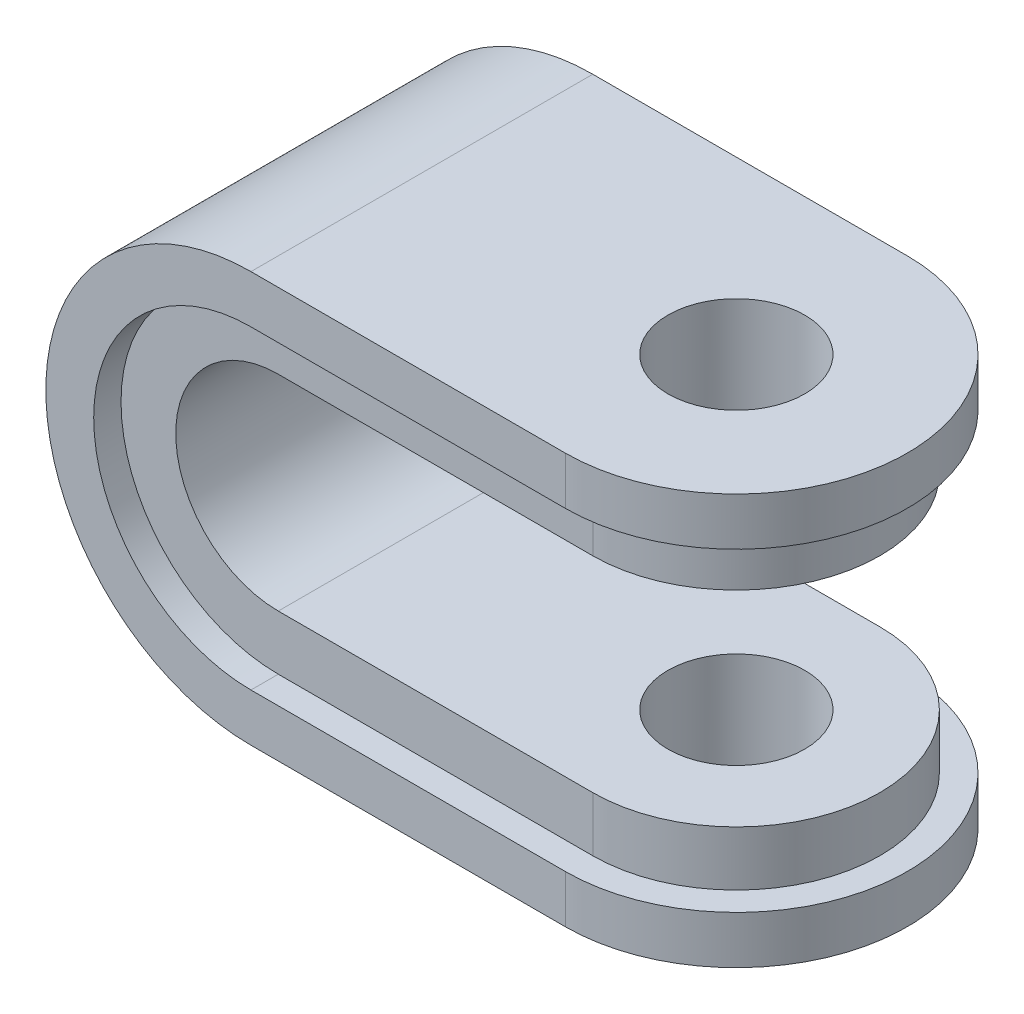
ISO-10303-21;
HEADER;
FILE_DESCRIPTION(('STEP AP214'),'2;1');
FILE_NAME('part.step','',(''),(''),'','','');
FILE_SCHEMA(('AUTOMOTIVE_DESIGN { 1 0 10303 214 1 1 1 1 }'));
ENDSEC;
DATA;
#1=APPLICATION_CONTEXT('core data for automotive mechanical design processes');
#2=APPLICATION_PROTOCOL_DEFINITION('international standard','automotive_design',2000,#1);
#3=PRODUCT_CONTEXT('',#1,'mechanical');
#4=PRODUCT('Part','Part','',(#3));
#5=PRODUCT_RELATED_PRODUCT_CATEGORY('part','',(#4));
#6=PRODUCT_DEFINITION_FORMATION('','',#4);
#7=PRODUCT_DEFINITION_CONTEXT('part definition',#1,'design');
#8=PRODUCT_DEFINITION('design','',#6,#7);
#9=PRODUCT_DEFINITION_SHAPE('','',#8);
#10=(LENGTH_UNIT() NAMED_UNIT(*) SI_UNIT(.MILLI.,.METRE.));
#11=(NAMED_UNIT(*) PLANE_ANGLE_UNIT() SI_UNIT($,.RADIAN.));
#12=(NAMED_UNIT(*) SI_UNIT($,.STERADIAN.) SOLID_ANGLE_UNIT());
#13=UNCERTAINTY_MEASURE_WITH_UNIT(LENGTH_MEASURE(1.E-05),#10,'distance_accuracy_value','');
#14=(GEOMETRIC_REPRESENTATION_CONTEXT(3) GLOBAL_UNCERTAINTY_ASSIGNED_CONTEXT((#13)) GLOBAL_UNIT_ASSIGNED_CONTEXT((#10,
#11,#12)) REPRESENTATION_CONTEXT('',''));
#15=CARTESIAN_POINT('',(0.,0.,0.));
#16=DIRECTION('',(0.,0.,1.));
#17=DIRECTION('',(1.,0.,0.));
#18=AXIS2_PLACEMENT_3D('',#15,#16,#17);
#19=CARTESIAN_POINT('',(46.,8.,25.));
#20=DIRECTION('',(0.,-1.,0.));
#21=DIRECTION('',(0.,0.,-1.));
#22=AXIS2_PLACEMENT_3D('',#19,#20,#21);
#23=CYLINDRICAL_SURFACE('',#22,25.);
#24=DIRECTION('',(0.,-1.,0.));
#25=VECTOR('',#24,1.);
#26=CARTESIAN_POINT('',(46.,0.,0.));
#27=LINE('',#26,#25);
#28=CARTESIAN_POINT('',(46.,7.,0.));
#29=VERTEX_POINT('',#28);
#30=CARTESIAN_POINT('',(46.,0.,0.));
#31=VERTEX_POINT('',#30);
#32=EDGE_CURVE('E179',#29,#31,#27,.T.);
#33=ORIENTED_EDGE('',*,*,#32,.F.);
#34=CARTESIAN_POINT('',(46.,7.,25.));
#35=DIRECTION('',(0.,1.,0.));
#36=DIRECTION('',(0.,0.,1.));
#37=AXIS2_PLACEMENT_3D('',#34,#35,#36);
#38=CIRCLE('',#37,25.);
#39=CARTESIAN_POINT('',(46.,6.99999999999999,50.));
#40=VERTEX_POINT('',#39);
#41=EDGE_CURVE('E222',#40,#29,#38,.T.);
#42=ORIENTED_EDGE('',*,*,#41,.F.);
#43=DIRECTION('',(0.,-1.,0.));
#44=VECTOR('',#43,1.);
#45=CARTESIAN_POINT('',(46.,0.,50.));
#46=LINE('',#45,#44);
#47=CARTESIAN_POINT('',(46.,0.,50.));
#48=VERTEX_POINT('',#47);
#49=EDGE_CURVE('E187',#40,#48,#46,.T.);
#50=ORIENTED_EDGE('',*,*,#49,.T.);
#51=CARTESIAN_POINT('',(46.,0.,25.));
#52=DIRECTION('',(0.,-1.,0.));
#53=DIRECTION('',(0.,0.,-1.));
#54=AXIS2_PLACEMENT_3D('',#51,#52,#53);
#55=CIRCLE('',#54,25.);
#56=EDGE_CURVE('E225',#31,#48,#55,.T.);
#57=ORIENTED_EDGE('',*,*,#56,.F.);
#58=EDGE_LOOP('',(#33,#42,#50,#57));
#59=FACE_BOUND('',#58,.T.);
#60=ADVANCED_FACE('F56',(#59),#23,.T.);
#61=CARTESIAN_POINT('',(46.,52.,25.));
#62=DIRECTION('',(0.,1.,0.));
#63=DIRECTION('',(0.,0.,1.));
#64=AXIS2_PLACEMENT_3D('',#61,#62,#63);
#65=CYLINDRICAL_SURFACE('',#64,25.);
#66=DIRECTION('',(0.,-1.,0.));
#67=VECTOR('',#66,1.);
#68=CARTESIAN_POINT('',(46.,0.,50.));
#69=LINE('',#68,#67);
#70=CARTESIAN_POINT('',(46.,60.,50.));
#71=VERTEX_POINT('',#70);
#72=CARTESIAN_POINT('',(46.,53.,50.));
#73=VERTEX_POINT('',#72);
#74=EDGE_CURVE('E176',#71,#73,#69,.T.);
#75=ORIENTED_EDGE('',*,*,#74,.T.);
#76=CARTESIAN_POINT('',(46.,53.,25.));
#77=DIRECTION('',(0.,-1.,0.));
#78=DIRECTION('',(0.,0.,-1.));
#79=AXIS2_PLACEMENT_3D('',#76,#77,#78);
#80=CIRCLE('',#79,25.);
#81=CARTESIAN_POINT('',(46.,53.,0.));
#82=VERTEX_POINT('',#81);
#83=EDGE_CURVE('E639',#82,#73,#80,.T.);
#84=ORIENTED_EDGE('',*,*,#83,.F.);
#85=DIRECTION('',(0.,-1.,0.));
#86=VECTOR('',#85,1.);
#87=CARTESIAN_POINT('',(46.,0.,0.));
#88=LINE('',#87,#86);
#89=CARTESIAN_POINT('',(46.,60.,0.));
#90=VERTEX_POINT('',#89);
#91=EDGE_CURVE('E172',#90,#82,#88,.T.);
#92=ORIENTED_EDGE('',*,*,#91,.F.);
#93=CARTESIAN_POINT('',(46.,60.,25.));
#94=DIRECTION('',(0.,1.,0.));
#95=DIRECTION('',(0.,0.,1.));
#96=AXIS2_PLACEMENT_3D('',#93,#94,#95);
#97=CIRCLE('',#96,25.);
#98=EDGE_CURVE('E306',#71,#90,#97,.T.);
#99=ORIENTED_EDGE('',*,*,#98,.F.);
#100=EDGE_LOOP('',(#75,#84,#92,#99));
#101=FACE_BOUND('',#100,.T.);
#102=ADVANCED_FACE('F349',(#101),#65,.T.);
#103=CARTESIAN_POINT('',(46.,7.,25.));
#104=DIRECTION('',(0.,1.,0.));
#105=DIRECTION('',(0.,0.,1.));
#106=AXIS2_PLACEMENT_3D('',#103,#104,#105);
#107=CYLINDRICAL_SURFACE('',#106,21.);
#108=CARTESIAN_POINT('',(46.,15.,25.));
#109=DIRECTION('',(0.,1.,0.));
#110=DIRECTION('',(0.,0.,1.));
#111=AXIS2_PLACEMENT_3D('',#108,#109,#110);
#112=CIRCLE('',#111,21.);
#113=CARTESIAN_POINT('',(46.,15.,46.));
#114=VERTEX_POINT('',#113);
#115=CARTESIAN_POINT('',(46.,15.,4.));
#116=VERTEX_POINT('',#115);
#117=EDGE_CURVE('E303',#114,#116,#112,.T.);
#118=ORIENTED_EDGE('',*,*,#117,.F.);
#119=DIRECTION('',(0.,1.,0.));
#120=VECTOR('',#119,1.);
#121=CARTESIAN_POINT('',(46.,6.99999999999999,46.));
#122=LINE('',#121,#120);
#123=CARTESIAN_POINT('',(46.,7.,46.));
#124=VERTEX_POINT('',#123);
#125=EDGE_CURVE('E163',#124,#114,#122,.T.);
#126=ORIENTED_EDGE('',*,*,#125,.F.);
#127=CARTESIAN_POINT('',(46.,7.,25.));
#128=DIRECTION('',(0.,-1.,0.));
#129=DIRECTION('',(0.,0.,1.));
#130=AXIS2_PLACEMENT_3D('',#127,#128,#129);
#131=CIRCLE('',#130,21.);
#132=CARTESIAN_POINT('',(46.,7.,4.));
#133=VERTEX_POINT('',#132);
#134=EDGE_CURVE('E328',#133,#124,#131,.T.);
#135=ORIENTED_EDGE('',*,*,#134,.F.);
#136=DIRECTION('',(0.,-1.,0.));
#137=VECTOR('',#136,1.);
#138=CARTESIAN_POINT('',(46.,6.99999999999999,4.));
#139=LINE('',#138,#137);
#140=EDGE_CURVE('E317',#116,#133,#139,.T.);
#141=ORIENTED_EDGE('',*,*,#140,.F.);
#142=EDGE_LOOP('',(#118,#126,#135,#141));
#143=FACE_BOUND('',#142,.T.);
#144=ADVANCED_FACE('F332',(#143),#107,.T.);
#145=CARTESIAN_POINT('',(46.,53.,25.));
#146=DIRECTION('',(0.,-1.,0.));
#147=DIRECTION('',(0.,0.,-1.));
#148=AXIS2_PLACEMENT_3D('',#145,#146,#147);
#149=CYLINDRICAL_SURFACE('',#148,21.);
#150=CARTESIAN_POINT('',(46.,45.,25.));
#151=DIRECTION('',(0.,-1.,0.));
#152=DIRECTION('',(0.,0.,-1.));
#153=AXIS2_PLACEMENT_3D('',#150,#151,#152);
#154=CIRCLE('',#153,21.);
#155=CARTESIAN_POINT('',(46.,45.,4.));
#156=VERTEX_POINT('',#155);
#157=CARTESIAN_POINT('',(46.,45.,46.));
#158=VERTEX_POINT('',#157);
#159=EDGE_CURVE('E299',#156,#158,#154,.T.);
#160=ORIENTED_EDGE('',*,*,#159,.F.);
#161=DIRECTION('',(0.,-1.,0.));
#162=VECTOR('',#161,1.);
#163=CARTESIAN_POINT('',(46.,53.,4.));
#164=LINE('',#163,#162);
#165=CARTESIAN_POINT('',(46.,53.,4.));
#166=VERTEX_POINT('',#165);
#167=EDGE_CURVE('E288',#166,#156,#164,.T.);
#168=ORIENTED_EDGE('',*,*,#167,.F.);
#169=CARTESIAN_POINT('',(46.,53.,25.));
#170=DIRECTION('',(0.,1.,0.));
#171=DIRECTION('',(0.,0.,-1.));
#172=AXIS2_PLACEMENT_3D('',#169,#170,#171);
#173=CIRCLE('',#172,21.);
#174=CARTESIAN_POINT('',(46.,53.,46.));
#175=VERTEX_POINT('',#174);
#176=EDGE_CURVE('E297',#175,#166,#173,.T.);
#177=ORIENTED_EDGE('',*,*,#176,.F.);
#178=DIRECTION('',(0.,1.,0.));
#179=VECTOR('',#178,1.);
#180=CARTESIAN_POINT('',(46.,53.,46.));
#181=LINE('',#180,#179);
#182=EDGE_CURVE('E152',#158,#175,#181,.T.);
#183=ORIENTED_EDGE('',*,*,#182,.F.);
#184=EDGE_LOOP('',(#160,#168,#177,#183));
#185=FACE_BOUND('',#184,.T.);
#186=ADVANCED_FACE('F296',(#185),#149,.T.);
#187=CARTESIAN_POINT('',(0.,45.,0.));
#188=DIRECTION('',(0.,-1.,0.));
#189=DIRECTION('',(0.,0.,-1.));
#190=AXIS2_PLACEMENT_3D('',#187,#188,#189);
#191=PLANE('',#190);
#192=CARTESIAN_POINT('',(46.,45.,25.));
#193=DIRECTION('',(0.,-1.,0.));
#194=DIRECTION('',(0.,0.,-1.));
#195=AXIS2_PLACEMENT_3D('',#192,#193,#194);
#196=CIRCLE('',#195,10.);
#197=CARTESIAN_POINT('',(46.,45.,15.));
#198=VERTEX_POINT('',#197);
#199=EDGE_CURVE('E382',#198,#198,#196,.T.);
#200=ORIENTED_EDGE('',*,*,#199,.F.);
#201=EDGE_LOOP('',(#200));
#202=FACE_BOUND('',#201,.T.);
#203=ORIENTED_EDGE('',*,*,#159,.T.);
#204=DIRECTION('',(1.,0.,0.));
#205=VECTOR('',#204,1.);
#206=CARTESIAN_POINT('',(0.,45.,46.));
#207=LINE('',#206,#205);
#208=CARTESIAN_POINT('',(0.,45.,46.));
#209=VERTEX_POINT('',#208);
#210=EDGE_CURVE('E158',#209,#158,#207,.T.);
#211=ORIENTED_EDGE('',*,*,#210,.F.);
#212=DIRECTION('',(0.,0.,1.));
#213=VECTOR('',#212,1.);
#214=CARTESIAN_POINT('',(0.,45.,0.));
#215=LINE('',#214,#213);
#216=CARTESIAN_POINT('',(0.,45.,4.));
#217=VERTEX_POINT('',#216);
#218=EDGE_CURVE('E117',#217,#209,#215,.T.);
#219=ORIENTED_EDGE('',*,*,#218,.F.);
#220=DIRECTION('',(-1.,0.,0.));
#221=VECTOR('',#220,1.);
#222=CARTESIAN_POINT('',(46.,45.,4.));
#223=LINE('',#222,#221);
#224=EDGE_CURVE('E287',#156,#217,#223,.T.);
#225=ORIENTED_EDGE('',*,*,#224,.F.);
#226=EDGE_LOOP('',(#203,#211,#219,#225));
#227=FACE_BOUND('',#226,.T.);
#228=ADVANCED_FACE('F305',(#202,#227),#191,.T.);
#229=CARTESIAN_POINT('',(0.,30.,0.));
#230=DIRECTION('',(0.,0.,1.));
#231=DIRECTION('',(1.,0.,0.));
#232=AXIS2_PLACEMENT_3D('',#229,#230,#231);
#233=CYLINDRICAL_SURFACE('',#232,15.);
#234=DIRECTION('',(0.,0.,1.));
#235=VECTOR('',#234,1.);
#236=CARTESIAN_POINT('',(0.,15.,0.));
#237=LINE('',#236,#235);
#238=CARTESIAN_POINT('',(0.,15.,4.));
#239=VERTEX_POINT('',#238);
#240=CARTESIAN_POINT('',(0.,15.,46.));
#241=VERTEX_POINT('',#240);
#242=EDGE_CURVE('E92',#239,#241,#237,.T.);
#243=ORIENTED_EDGE('',*,*,#242,.F.);
#244=CARTESIAN_POINT('',(0.,30.,4.));
#245=DIRECTION('',(0.,0.,1.));
#246=DIRECTION('',(-1.,0.,0.));
#247=AXIS2_PLACEMENT_3D('',#244,#245,#246);
#248=CIRCLE('',#247,15.);
#249=EDGE_CURVE('E311',#217,#239,#248,.T.);
#250=ORIENTED_EDGE('',*,*,#249,.F.);
#251=ORIENTED_EDGE('',*,*,#218,.T.);
#252=CARTESIAN_POINT('',(0.,30.,46.));
#253=DIRECTION('',(0.,0.,-1.));
#254=DIRECTION('',(1.,0.,0.));
#255=AXIS2_PLACEMENT_3D('',#252,#253,#254);
#256=CIRCLE('',#255,15.);
#257=EDGE_CURVE('E171',#241,#209,#256,.T.);
#258=ORIENTED_EDGE('',*,*,#257,.F.);
#259=EDGE_LOOP('',(#243,#250,#251,#258));
#260=FACE_BOUND('',#259,.T.);
#261=ADVANCED_FACE('F337',(#260),#233,.F.);
#262=CARTESIAN_POINT('',(0.,15.,0.));
#263=DIRECTION('',(0.,1.,0.));
#264=DIRECTION('',(0.,0.,1.));
#265=AXIS2_PLACEMENT_3D('',#262,#263,#264);
#266=PLANE('',#265);
#267=CARTESIAN_POINT('',(46.,15.,25.));
#268=DIRECTION('',(0.,1.,0.));
#269=DIRECTION('',(0.,0.,1.));
#270=AXIS2_PLACEMENT_3D('',#267,#268,#269);
#271=CIRCLE('',#270,10.);
#272=CARTESIAN_POINT('',(46.,15.,35.));
#273=VERTEX_POINT('',#272);
#274=EDGE_CURVE('E384',#273,#273,#271,.T.);
#275=ORIENTED_EDGE('',*,*,#274,.F.);
#276=EDGE_LOOP('',(#275));
#277=FACE_BOUND('',#276,.T.);
#278=DIRECTION('',(-1.,0.,0.));
#279=VECTOR('',#278,1.);
#280=CARTESIAN_POINT('',(0.,15.,46.));
#281=LINE('',#280,#279);
#282=EDGE_CURVE('E142',#114,#241,#281,.T.);
#283=ORIENTED_EDGE('',*,*,#282,.F.);
#284=ORIENTED_EDGE('',*,*,#117,.T.);
#285=DIRECTION('',(1.,0.,0.));
#286=VECTOR('',#285,1.);
#287=CARTESIAN_POINT('',(46.,15.,4.));
#288=LINE('',#287,#286);
#289=EDGE_CURVE('E312',#239,#116,#288,.T.);
#290=ORIENTED_EDGE('',*,*,#289,.F.);
#291=ORIENTED_EDGE('',*,*,#242,.T.);
#292=EDGE_LOOP('',(#283,#284,#290,#291));
#293=FACE_BOUND('',#292,.T.);
#294=ADVANCED_FACE('F335',(#277,#293),#266,.T.);
#295=CARTESIAN_POINT('',(0.,60.,50.));
#296=DIRECTION('',(0.,1.,0.));
#297=DIRECTION('',(0.,0.,1.));
#298=AXIS2_PLACEMENT_3D('',#295,#296,#297);
#299=PLANE('',#298);
#300=CARTESIAN_POINT('',(46.,60.,25.));
#301=DIRECTION('',(0.,1.,0.));
#302=DIRECTION('',(0.,0.,1.));
#303=AXIS2_PLACEMENT_3D('',#300,#301,#302);
#304=CIRCLE('',#303,10.);
#305=CARTESIAN_POINT('',(46.,60.,35.));
#306=VERTEX_POINT('',#305);
#307=EDGE_CURVE('E390',#306,#306,#304,.T.);
#308=ORIENTED_EDGE('',*,*,#307,.F.);
#309=EDGE_LOOP('',(#308));
#310=FACE_BOUND('',#309,.T.);
#311=DIRECTION('',(1.,0.,0.));
#312=VECTOR('',#311,1.);
#313=CARTESIAN_POINT('',(0.,60.,0.));
#314=LINE('',#313,#312);
#315=CARTESIAN_POINT('',(0.,60.,0.));
#316=VERTEX_POINT('',#315);
#317=EDGE_CURVE('E191',#316,#90,#314,.T.);
#318=ORIENTED_EDGE('',*,*,#317,.F.);
#319=DIRECTION('',(0.,0.,-1.));
#320=VECTOR('',#319,1.);
#321=CARTESIAN_POINT('',(0.,60.,50.));
#322=LINE('',#321,#320);
#323=CARTESIAN_POINT('',(0.,60.,50.));
#324=VERTEX_POINT('',#323);
#325=EDGE_CURVE('E12',#324,#316,#322,.T.);
#326=ORIENTED_EDGE('',*,*,#325,.F.);
#327=DIRECTION('',(1.,0.,0.));
#328=VECTOR('',#327,1.);
#329=CARTESIAN_POINT('',(0.,60.,50.));
#330=LINE('',#329,#328);
#331=EDGE_CURVE('E177',#324,#71,#330,.T.);
#332=ORIENTED_EDGE('',*,*,#331,.T.);
#333=ORIENTED_EDGE('',*,*,#98,.T.);
#334=EDGE_LOOP('',(#318,#326,#332,#333));
#335=FACE_BOUND('',#334,.T.);
#336=ADVANCED_FACE('F61',(#310,#335),#299,.T.);
#337=CARTESIAN_POINT('',(0.,30.,50.));
#338=DIRECTION('',(0.,0.,-1.));
#339=DIRECTION('',(-1.,0.,0.));
#340=AXIS2_PLACEMENT_3D('',#337,#338,#339);
#341=CYLINDRICAL_SURFACE('',#340,30.);
#342=CARTESIAN_POINT('',(0.,30.,0.));
#343=DIRECTION('',(0.,0.,1.));
#344=DIRECTION('',(1.,0.,0.));
#345=AXIS2_PLACEMENT_3D('',#342,#343,#344);
#346=CIRCLE('',#345,30.);
#347=CARTESIAN_POINT('',(0.,0.,0.));
#348=VERTEX_POINT('',#347);
#349=EDGE_CURVE('E193',#316,#348,#346,.T.);
#350=ORIENTED_EDGE('',*,*,#349,.T.);
#351=DIRECTION('',(0.,0.,-1.));
#352=VECTOR('',#351,1.);
#353=CARTESIAN_POINT('',(0.,0.,50.));
#354=LINE('',#353,#352);
#355=CARTESIAN_POINT('',(0.,0.,50.));
#356=VERTEX_POINT('',#355);
#357=EDGE_CURVE('E67',#356,#348,#354,.T.);
#358=ORIENTED_EDGE('',*,*,#357,.F.);
#359=CARTESIAN_POINT('',(0.,30.,50.));
#360=DIRECTION('',(0.,0.,1.));
#361=DIRECTION('',(1.,0.,0.));
#362=AXIS2_PLACEMENT_3D('',#359,#360,#361);
#363=CIRCLE('',#362,30.);
#364=EDGE_CURVE('E77',#324,#356,#363,.T.);
#365=ORIENTED_EDGE('',*,*,#364,.F.);
#366=ORIENTED_EDGE('',*,*,#325,.T.);
#367=EDGE_LOOP('',(#350,#358,#365,#366));
#368=FACE_BOUND('',#367,.T.);
#369=ADVANCED_FACE('F342',(#368),#341,.T.);
#370=CARTESIAN_POINT('',(0.,0.,50.));
#371=DIRECTION('',(0.,1.,0.));
#372=DIRECTION('',(0.,0.,1.));
#373=AXIS2_PLACEMENT_3D('',#370,#371,#372);
#374=PLANE('',#373);
#375=CARTESIAN_POINT('',(46.,0.,25.));
#376=DIRECTION('',(0.,-1.,0.));
#377=DIRECTION('',(0.,0.,-1.));
#378=AXIS2_PLACEMENT_3D('',#375,#376,#377);
#379=CIRCLE('',#378,10.);
#380=CARTESIAN_POINT('',(46.,0.,15.));
#381=VERTEX_POINT('',#380);
#382=EDGE_CURVE('E637',#381,#381,#379,.T.);
#383=ORIENTED_EDGE('',*,*,#382,.F.);
#384=EDGE_LOOP('',(#383));
#385=FACE_BOUND('',#384,.T.);
#386=DIRECTION('',(1.,0.,0.));
#387=VECTOR('',#386,1.);
#388=CARTESIAN_POINT('',(0.,0.,0.));
#389=LINE('',#388,#387);
#390=EDGE_CURVE('E196',#348,#31,#389,.T.);
#391=ORIENTED_EDGE('',*,*,#390,.T.);
#392=ORIENTED_EDGE('',*,*,#56,.T.);
#393=DIRECTION('',(1.,0.,0.));
#394=VECTOR('',#393,1.);
#395=CARTESIAN_POINT('',(0.,0.,50.));
#396=LINE('',#395,#394);
#397=EDGE_CURVE('E183',#356,#48,#396,.T.);
#398=ORIENTED_EDGE('',*,*,#397,.F.);
#399=ORIENTED_EDGE('',*,*,#357,.T.);
#400=EDGE_LOOP('',(#391,#392,#398,#399));
#401=FACE_BOUND('',#400,.T.);
#402=ADVANCED_FACE('F205',(#385,#401),#374,.F.);
#403=CARTESIAN_POINT('',(0.,0.,50.));
#404=DIRECTION('',(0.,0.,1.));
#405=DIRECTION('',(1.,0.,0.));
#406=AXIS2_PLACEMENT_3D('',#403,#404,#405);
#407=PLANE('',#406);
#408=DIRECTION('',(1.,0.,0.));
#409=VECTOR('',#408,1.);
#410=CARTESIAN_POINT('',(2.40912212380176E-13,6.99999999999999,50.));
#411=LINE('',#410,#409);
#412=CARTESIAN_POINT('',(2.40912212380176E-13,6.99999999999999,50.));
#413=VERTEX_POINT('',#412);
#414=EDGE_CURVE('E169',#413,#40,#411,.T.);
#415=ORIENTED_EDGE('',*,*,#414,.F.);
#416=CARTESIAN_POINT('',(0.,30.,50.));
#417=DIRECTION('',(0.,0.,1.));
#418=DIRECTION('',(1.,0.,0.));
#419=AXIS2_PLACEMENT_3D('',#416,#417,#418);
#420=CIRCLE('',#419,23.);
#421=CARTESIAN_POINT('',(0.,53.,50.));
#422=VERTEX_POINT('',#421);
#423=EDGE_CURVE('E168',#422,#413,#420,.T.);
#424=ORIENTED_EDGE('',*,*,#423,.F.);
#425=DIRECTION('',(-1.,0.,0.));
#426=VECTOR('',#425,1.);
#427=CARTESIAN_POINT('',(0.,53.,50.));
#428=LINE('',#427,#426);
#429=EDGE_CURVE('E137',#73,#422,#428,.T.);
#430=ORIENTED_EDGE('',*,*,#429,.F.);
#431=ORIENTED_EDGE('',*,*,#74,.F.);
#432=ORIENTED_EDGE('',*,*,#331,.F.);
#433=ORIENTED_EDGE('',*,*,#364,.T.);
#434=ORIENTED_EDGE('',*,*,#397,.T.);
#435=ORIENTED_EDGE('',*,*,#49,.F.);
#436=EDGE_LOOP('',(#415,#424,#430,#431,#432,#433,#434,#435));
#437=FACE_BOUND('',#436,.T.);
#438=ADVANCED_FACE('F393',(#437),#407,.T.);
#439=CARTESIAN_POINT('',(0.,0.,0.));
#440=DIRECTION('',(0.,0.,1.));
#441=DIRECTION('',(1.,0.,0.));
#442=AXIS2_PLACEMENT_3D('',#439,#440,#441);
#443=PLANE('',#442);
#444=ORIENTED_EDGE('',*,*,#91,.T.);
#445=DIRECTION('',(1.,0.,0.));
#446=VECTOR('',#445,1.);
#447=CARTESIAN_POINT('',(0.,53.,0.));
#448=LINE('',#447,#446);
#449=CARTESIAN_POINT('',(0.,53.,0.));
#450=VERTEX_POINT('',#449);
#451=EDGE_CURVE('E277',#450,#82,#448,.T.);
#452=ORIENTED_EDGE('',*,*,#451,.F.);
#453=CARTESIAN_POINT('',(0.,30.,0.));
#454=DIRECTION('',(0.,0.,-1.));
#455=DIRECTION('',(-1.,0.,0.));
#456=AXIS2_PLACEMENT_3D('',#453,#454,#455);
#457=CIRCLE('',#456,23.);
#458=CARTESIAN_POINT('',(0.,7.00000000000001,0.));
#459=VERTEX_POINT('',#458);
#460=EDGE_CURVE('E282',#459,#450,#457,.T.);
#461=ORIENTED_EDGE('',*,*,#460,.F.);
#462=DIRECTION('',(-1.,0.,0.));
#463=VECTOR('',#462,1.);
#464=CARTESIAN_POINT('',(0.,7.00000000000001,0.));
#465=LINE('',#464,#463);
#466=EDGE_CURVE('E214',#29,#459,#465,.T.);
#467=ORIENTED_EDGE('',*,*,#466,.F.);
#468=ORIENTED_EDGE('',*,*,#32,.T.);
#469=ORIENTED_EDGE('',*,*,#390,.F.);
#470=ORIENTED_EDGE('',*,*,#349,.F.);
#471=ORIENTED_EDGE('',*,*,#317,.T.);
#472=EDGE_LOOP('',(#444,#452,#461,#467,#468,#469,#470,#471));
#473=FACE_BOUND('',#472,.T.);
#474=ADVANCED_FACE('F206',(#473),#443,.F.);
#475=CARTESIAN_POINT('',(2.40912212380176E-13,6.99999999999999,46.));
#476=DIRECTION('',(0.,-1.,0.));
#477=DIRECTION('',(1.,0.,0.));
#478=AXIS2_PLACEMENT_3D('',#475,#476,#477);
#479=PLANE('',#478);
#480=ORIENTED_EDGE('',*,*,#414,.T.);
#481=ORIENTED_EDGE('',*,*,#41,.T.);
#482=ORIENTED_EDGE('',*,*,#466,.T.);
#483=DIRECTION('',(0.,0.,-1.));
#484=VECTOR('',#483,1.);
#485=CARTESIAN_POINT('',(0.,7.00000000000001,4.));
#486=LINE('',#485,#484);
#487=CARTESIAN_POINT('',(0.,7.00000000000001,4.));
#488=VERTEX_POINT('',#487);
#489=EDGE_CURVE('E271',#488,#459,#486,.T.);
#490=ORIENTED_EDGE('',*,*,#489,.F.);
#491=DIRECTION('',(-1.,0.,0.));
#492=VECTOR('',#491,1.);
#493=CARTESIAN_POINT('',(0.,7.00000000000001,4.));
#494=LINE('',#493,#492);
#495=EDGE_CURVE('E319',#133,#488,#494,.T.);
#496=ORIENTED_EDGE('',*,*,#495,.F.);
#497=ORIENTED_EDGE('',*,*,#134,.T.);
#498=DIRECTION('',(1.,0.,0.));
#499=VECTOR('',#498,1.);
#500=CARTESIAN_POINT('',(2.40912212380176E-13,6.99999999999999,46.));
#501=LINE('',#500,#499);
#502=CARTESIAN_POINT('',(2.40912212380176E-13,6.99999999999999,46.));
#503=VERTEX_POINT('',#502);
#504=EDGE_CURVE('E147',#503,#124,#501,.T.);
#505=ORIENTED_EDGE('',*,*,#504,.F.);
#506=DIRECTION('',(0.,0.,1.));
#507=VECTOR('',#506,1.);
#508=CARTESIAN_POINT('',(2.40912212380176E-13,6.99999999999999,46.));
#509=LINE('',#508,#507);
#510=EDGE_CURVE('E107',#503,#413,#509,.T.);
#511=ORIENTED_EDGE('',*,*,#510,.T.);
#512=EDGE_LOOP('',(#480,#481,#482,#490,#496,#497,#505,#511));
#513=FACE_BOUND('',#512,.T.);
#514=ADVANCED_FACE('F327',(#513),#479,.F.);
#515=CARTESIAN_POINT('',(0.,30.,46.));
#516=DIRECTION('',(0.,0.,1.));
#517=DIRECTION('',(1.,0.,0.));
#518=AXIS2_PLACEMENT_3D('',#515,#516,#517);
#519=CYLINDRICAL_SURFACE('',#518,23.);
#520=ORIENTED_EDGE('',*,*,#423,.T.);
#521=ORIENTED_EDGE('',*,*,#510,.F.);
#522=CARTESIAN_POINT('',(0.,30.,46.));
#523=DIRECTION('',(0.,0.,1.));
#524=DIRECTION('',(1.,0.,0.));
#525=AXIS2_PLACEMENT_3D('',#522,#523,#524);
#526=CIRCLE('',#525,23.);
#527=CARTESIAN_POINT('',(0.,53.,46.));
#528=VERTEX_POINT('',#527);
#529=EDGE_CURVE('E144',#528,#503,#526,.T.);
#530=ORIENTED_EDGE('',*,*,#529,.F.);
#531=DIRECTION('',(0.,0.,1.));
#532=VECTOR('',#531,1.);
#533=CARTESIAN_POINT('',(0.,53.,46.));
#534=LINE('',#533,#532);
#535=EDGE_CURVE('E128',#528,#422,#534,.T.);
#536=ORIENTED_EDGE('',*,*,#535,.T.);
#537=EDGE_LOOP('',(#520,#521,#530,#536));
#538=FACE_BOUND('',#537,.T.);
#539=ADVANCED_FACE('F143',(#538),#519,.F.);
#540=CARTESIAN_POINT('',(0.,53.,46.));
#541=DIRECTION('',(0.,1.,0.));
#542=DIRECTION('',(0.,0.,1.));
#543=AXIS2_PLACEMENT_3D('',#540,#541,#542);
#544=PLANE('',#543);
#545=ORIENTED_EDGE('',*,*,#429,.T.);
#546=ORIENTED_EDGE('',*,*,#535,.F.);
#547=DIRECTION('',(-1.,0.,0.));
#548=VECTOR('',#547,1.);
#549=CARTESIAN_POINT('',(0.,53.,46.));
#550=LINE('',#549,#548);
#551=EDGE_CURVE('E134',#175,#528,#550,.T.);
#552=ORIENTED_EDGE('',*,*,#551,.F.);
#553=ORIENTED_EDGE('',*,*,#176,.T.);
#554=DIRECTION('',(1.,0.,0.));
#555=VECTOR('',#554,1.);
#556=CARTESIAN_POINT('',(0.,53.,4.));
#557=LINE('',#556,#555);
#558=CARTESIAN_POINT('',(0.,53.,4.));
#559=VERTEX_POINT('',#558);
#560=EDGE_CURVE('E279',#559,#166,#557,.T.);
#561=ORIENTED_EDGE('',*,*,#560,.F.);
#562=DIRECTION('',(0.,0.,-1.));
#563=VECTOR('',#562,1.);
#564=CARTESIAN_POINT('',(0.,53.,4.));
#565=LINE('',#564,#563);
#566=EDGE_CURVE('E170',#559,#450,#565,.T.);
#567=ORIENTED_EDGE('',*,*,#566,.T.);
#568=ORIENTED_EDGE('',*,*,#451,.T.);
#569=ORIENTED_EDGE('',*,*,#83,.T.);
#570=EDGE_LOOP('',(#545,#546,#552,#553,#561,#567,#568,#569));
#571=FACE_BOUND('',#570,.T.);
#572=ADVANCED_FACE('F131',(#571),#544,.F.);
#573=CARTESIAN_POINT('',(0.,30.,46.));
#574=DIRECTION('',(0.,0.,1.));
#575=DIRECTION('',(1.,0.,0.));
#576=AXIS2_PLACEMENT_3D('',#573,#574,#575);
#577=PLANE('',#576);
#578=ORIENTED_EDGE('',*,*,#257,.T.);
#579=ORIENTED_EDGE('',*,*,#210,.T.);
#580=ORIENTED_EDGE('',*,*,#182,.T.);
#581=ORIENTED_EDGE('',*,*,#551,.T.);
#582=ORIENTED_EDGE('',*,*,#529,.T.);
#583=ORIENTED_EDGE('',*,*,#504,.T.);
#584=ORIENTED_EDGE('',*,*,#125,.T.);
#585=ORIENTED_EDGE('',*,*,#282,.T.);
#586=EDGE_LOOP('',(#578,#579,#580,#581,#582,#583,#584,#585));
#587=FACE_BOUND('',#586,.T.);
#588=ADVANCED_FACE('F151',(#587),#577,.T.);
#589=CARTESIAN_POINT('',(0.,30.,4.));
#590=DIRECTION('',(0.,0.,-1.));
#591=DIRECTION('',(-1.,0.,0.));
#592=AXIS2_PLACEMENT_3D('',#589,#590,#591);
#593=CYLINDRICAL_SURFACE('',#592,23.);
#594=ORIENTED_EDGE('',*,*,#460,.T.);
#595=ORIENTED_EDGE('',*,*,#566,.F.);
#596=CARTESIAN_POINT('',(0.,30.,4.));
#597=DIRECTION('',(0.,0.,-1.));
#598=DIRECTION('',(-1.,0.,0.));
#599=AXIS2_PLACEMENT_3D('',#596,#597,#598);
#600=CIRCLE('',#599,23.);
#601=EDGE_CURVE('E321',#488,#559,#600,.T.);
#602=ORIENTED_EDGE('',*,*,#601,.F.);
#603=ORIENTED_EDGE('',*,*,#489,.T.);
#604=EDGE_LOOP('',(#594,#595,#602,#603));
#605=FACE_BOUND('',#604,.T.);
#606=ADVANCED_FACE('F283',(#605),#593,.F.);
#607=CARTESIAN_POINT('',(0.,30.,4.));
#608=DIRECTION('',(0.,0.,-1.));
#609=DIRECTION('',(-1.,0.,0.));
#610=AXIS2_PLACEMENT_3D('',#607,#608,#609);
#611=PLANE('',#610);
#612=ORIENTED_EDGE('',*,*,#167,.T.);
#613=ORIENTED_EDGE('',*,*,#224,.T.);
#614=ORIENTED_EDGE('',*,*,#249,.T.);
#615=ORIENTED_EDGE('',*,*,#289,.T.);
#616=ORIENTED_EDGE('',*,*,#140,.T.);
#617=ORIENTED_EDGE('',*,*,#495,.T.);
#618=ORIENTED_EDGE('',*,*,#601,.T.);
#619=ORIENTED_EDGE('',*,*,#560,.T.);
#620=EDGE_LOOP('',(#612,#613,#614,#615,#616,#617,#618,#619));
#621=FACE_BOUND('',#620,.T.);
#622=ADVANCED_FACE('F323',(#621),#611,.T.);
#623=CARTESIAN_POINT('',(46.,70.,25.));
#624=DIRECTION('',(0.,-1.,0.));
#625=DIRECTION('',(0.,0.,-1.));
#626=AXIS2_PLACEMENT_3D('',#623,#624,#625);
#627=CYLINDRICAL_SURFACE('',#626,10.);
#628=ORIENTED_EDGE('',*,*,#274,.T.);
#629=EDGE_LOOP('',(#628));
#630=FACE_BOUND('',#629,.T.);
#631=ORIENTED_EDGE('',*,*,#382,.T.);
#632=EDGE_LOOP('',(#631));
#633=FACE_BOUND('',#632,.T.);
#634=ADVANCED_FACE('F356',(#630,#633),#627,.F.);
#635=ORIENTED_EDGE('',*,*,#199,.T.);
#636=EDGE_LOOP('',(#635));
#637=FACE_BOUND('',#636,.T.);
#638=ORIENTED_EDGE('',*,*,#307,.T.);
#639=EDGE_LOOP('',(#638));
#640=FACE_BOUND('',#639,.T.);
#641=ADVANCED_FACE('F482',(#637,#640),#627,.F.);
#642=CLOSED_SHELL('',(#60,#102,#144,#186,#228,#261,#294,#336,#369,#402,#438,#474,#514,#539,#572,
#588,#606,#622,#634,#641));
#643=MANIFOLD_SOLID_BREP('B2',#642);
#644=ADVANCED_BREP_SHAPE_REPRESENTATION('',(#18,#643),#14);
#645=SHAPE_DEFINITION_REPRESENTATION(#9,#644);
ENDSEC;
END-ISO-10303-21;
